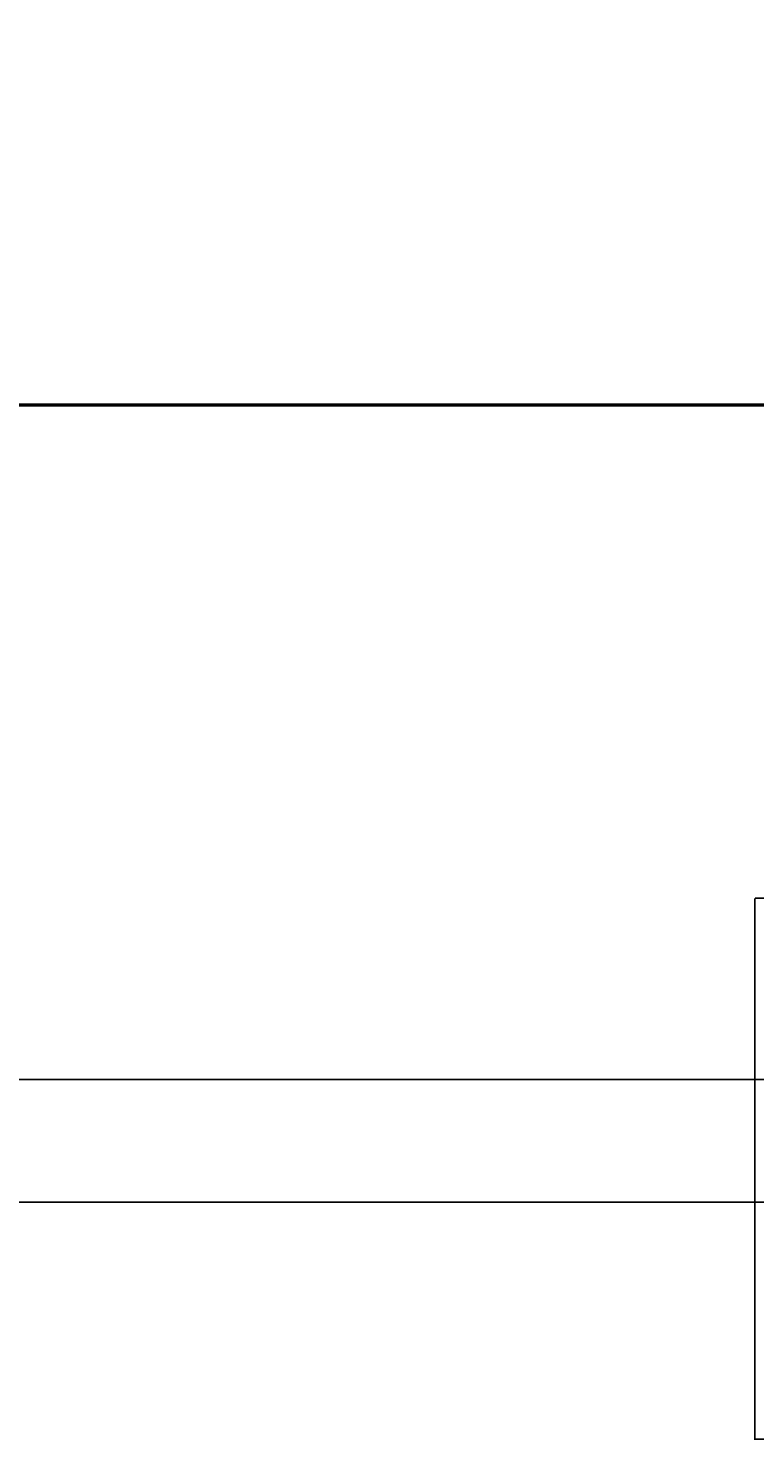
# Model space of a CAD drawing. Units: inches. Extents: x 1693 to 2974, y 2201 to 2965.
# Tile 11 of 24: x 2299 to 2479, y 2201 to 2550. Entities that reach past the tile are written whole.
import ezdxf

# ---------------------------------------------------------------- set-up
doc = ezdxf.new("R2010")
doc.units = ezdxf.units.IN
doc.header["$LTSCALE"] = 2
doc.header["$MEASUREMENT"] = 0
doc.layers.add('A-ANNO-DIMS', color=2, linetype='Continuous', lineweight=18)
doc.styles.get("Standard").update_dxf_attribs({"font": 'arial.ttf'})
doc.dimstyles.get("Standard").update_dxf_attribs({"dimtxt": 0.18, "dimasz": 0.18, "dimexe": 0.18, "dimexo": 0.0625, "dimgap": 0.09, "dimtad": 0, "dimtih": 1, "dimtoh": 1, "dimdec": 1, "dimzin": 0, "dimdsep": 46, "dimlunit": 3, "dimtxsty": 'Standard', "dimcen": 0.09, "dimadec": 0, "dimazin": 0, "dimtfac": 1, "dimtdec": 1, "dimtofl": 0, "dimtmove": 0, "dimatfit": 3, "dimfxl": 1, "dimtolj": 1, "dimtzin": 0, "dimarcsym": 0})

# ---------------------------------------------------------------- blocks, each defined once
blk = doc.blocks.new('*D82')
at = {"layer": 'A-ANNO-DIMS', "color": 0, "lineweight": -2, "ltscale": 2, "transparency": 16777216}
for p, q in [((2615.67, 2906.08), (1693.46, 2906.08)), ((1693.64, 2905.9), (1693.64, 2582.94)), ((1693.64, 2259.62), (1693.64, 2582.58)), ((2096.17, 2259.44), (1693.46, 2259.44))]:
    blk.add_line(p, q, dxfattribs=at)
at = {"layer": 'A-ANNO-DIMS', "color": 0, "ltscale": 2, "transparency": 16777216}
for points in [[(1693.61, 2905.9), (1693.67, 2905.9), (1693.64, 2906.08)], [(1693.61, 2259.62), (1693.67, 2259.62), (1693.64, 2259.44)]]:
    blk.add_solid(points, dxfattribs=at)
at = {"layer": 'Defpoints', "color": 0, "ltscale": 2, "transparency": 16777216}
for p in [(1693.64, 2906.08), (2615.74, 2906.08), (2096.24, 2259.44)]:
    blk.add_point(p, dxfattribs=at)
at = {"layer": 'A-ANNO-DIMS', "color": 0, "ltscale": 2, "transparency": 16777216, "insert": (1693.64, 2582.76), "char_height": 0.18, "attachment_point": 5}
blk.add_mtext('\\A1;646.6', dxfattribs=at)
blk = doc.blocks.new('*D85')
at = {"layer": 'A-ANNO-DIMS', "color": 0, "lineweight": -2, "ltscale": 2, "transparency": 16777216}
for p, q in [((2479.24, 2334.69), (2479.24, 2200.56)), ((2902.24, 2334.69), (2902.24, 2200.56)), ((2479.42, 2200.74), (2690.44, 2200.74)), ((2902.06, 2200.74), (2691.03, 2200.74))]:
    blk.add_line(p, q, dxfattribs=at)
at = {"layer": 'A-ANNO-DIMS', "color": 0, "ltscale": 2, "transparency": 16777216}
for points in [[(2479.42, 2200.77), (2479.42, 2200.71), (2479.24, 2200.74)], [(2902.06, 2200.77), (2902.06, 2200.71), (2902.24, 2200.74)]]:
    blk.add_solid(points, dxfattribs=at)
at = {"layer": 'Defpoints', "color": 0, "ltscale": 2, "transparency": 16777216}
for p in [(2479.24, 2334.75), (2902.24, 2334.75), (2902.24, 2200.74)]:
    blk.add_point(p, dxfattribs=at)
at = {"layer": 'A-ANNO-DIMS', "color": 0, "ltscale": 2, "transparency": 16777216, "insert": (2690.74, 2200.74), "char_height": 0.18, "attachment_point": 5}
blk.add_mtext('\\A1;423', dxfattribs=at)
blk = doc.blocks.new('*D89')
at = {"layer": 'A-ANNO-DIMS', "color": 0, "lineweight": -2, "ltscale": 2, "transparency": 16777216}
for p, q in [((2479.3, 2334.75), (2973.12, 2334.75)), ((2972.94, 2334.57), (2972.94, 2312.48)), ((2972.94, 2290.02), (2972.94, 2312.12)), ((2294.3, 2289.84), (2973.12, 2289.84))]:
    blk.add_line(p, q, dxfattribs=at)
at = {"layer": 'A-ANNO-DIMS', "color": 0, "ltscale": 2, "transparency": 16777216}
for points in [[(2972.91, 2334.57), (2972.97, 2334.57), (2972.94, 2334.75)], [(2972.91, 2290.02), (2972.97, 2290.02), (2972.94, 2289.84)]]:
    blk.add_solid(points, dxfattribs=at)
at = {"layer": 'Defpoints', "color": 0, "ltscale": 2, "transparency": 16777216}
for p in [(2479.24, 2334.75), (2972.94, 2334.75), (2294.24, 2289.84)]:
    blk.add_point(p, dxfattribs=at)
at = {"layer": 'A-ANNO-DIMS', "color": 0, "ltscale": 2, "transparency": 16777216, "insert": (2972.94, 2312.3), "char_height": 0.18, "attachment_point": 5}
blk.add_mtext('\\A1;44.91', dxfattribs=at)
blk = doc.blocks.new('*D95')
at = {"layer": 'A-ANNO-DIMS', "color": 0, "lineweight": -2, "ltscale": 2, "transparency": 16777216}
for p, q in [((2189.3, 2289.84), (2973.12, 2289.84)), ((2972.94, 2289.66), (2972.94, 2274.83)), ((2972.94, 2259.62), (2972.94, 2274.46)), ((2189.3, 2259.44), (2973.12, 2259.44))]:
    blk.add_line(p, q, dxfattribs=at)
at = {"layer": 'A-ANNO-DIMS', "color": 0, "ltscale": 2, "transparency": 16777216}
for points in [[(2972.91, 2289.66), (2972.97, 2289.66), (2972.94, 2289.84)], [(2972.91, 2259.62), (2972.97, 2259.62), (2972.94, 2259.44)]]:
    blk.add_solid(points, dxfattribs=at)
at = {"layer": 'Defpoints', "color": 0, "ltscale": 2, "transparency": 16777216}
for p in [(2189.24, 2289.84), (2972.94, 2289.84), (2189.24, 2259.44)]:
    blk.add_point(p, dxfattribs=at)
at = {"layer": 'A-ANNO-DIMS', "color": 0, "ltscale": 2, "transparency": 16777216, "insert": (2972.94, 2274.64), "char_height": 0.18, "attachment_point": 5}
blk.add_mtext('\\A1;30.4', dxfattribs=at)
blk = doc.blocks.new('*D108')
at = {"layer": 'A-ANNO-DIMS', "color": 0, "lineweight": -2, "ltscale": 2, "transparency": 16777216}
for p, q in [((1752.74, 2457.09), (2973.12, 2457.09)), ((1752.74, 2456.73), (2973.12, 2456.73)), ((2972.94, 2457.27), (2972.94, 2457.45)), ((2972.94, 2457.45), (2973.12, 2457.45)), ((2972.94, 2456.55), (2972.94, 2456.37))]:
    blk.add_line(p, q, dxfattribs=at)
at = {"layer": 'A-ANNO-DIMS', "color": 0, "ltscale": 2, "transparency": 16777216}
for points in [[(2972.91, 2457.27), (2972.97, 2457.27), (2972.94, 2457.09)], [(2972.91, 2456.55), (2972.97, 2456.55), (2972.94, 2456.73)]]:
    blk.add_solid(points, dxfattribs=at)
at = {"layer": 'Defpoints', "color": 0, "ltscale": 2, "transparency": 16777216}
for p in [(1752.68, 2457.09), (1752.68, 2456.73), (2972.94, 2457.09)]:
    blk.add_point(p, dxfattribs=at)
at = {"layer": 'A-ANNO-DIMS', "color": 0, "ltscale": 2, "transparency": 16777216, "insert": (2973.44, 2457.45), "char_height": 0.18, "attachment_point": 5}
blk.add_mtext('\\A1;0.36', dxfattribs=at)

msp = doc.modelspace()

# ---------------------------------------------------------------- dimensions: what is measured, and where the dimension line sits
at = {"layer": 'A-ANNO-DIMS', "ltscale": 2}
for base, p1, p2, override, picture, middle in [((1693.6363, 2906.0761), (2096.2363, 2259.4449), (2615.7363, 2906.0761), {"dimdec": 1, "dimlfac": 1, "dimrnd": 0, "dimzin": 0, "dimdsep": 46, "dimlunit": 2}, '*D82', (1693.6363, 2582.7605)), ((2972.9363, 2457.0877), (1752.6754, 2456.7302), (1752.6754, 2457.0877), {"dimdec": 2, "dimlfac": 1, "dimrnd": 0, "dimzin": 0, "dimdsep": 46, "dimlunit": 2}, '*D108', (2973.44, 2457.4477)), ((2972.9363, 2334.7547), (2294.2363, 2289.8449), (2479.2363, 2334.7547), {"dimdec": 2, "dimlfac": 1, "dimrnd": 0, "dimzin": 0, "dimdsep": 46, "dimlunit": 2}, '*D89', (2972.9363, 2312.2998)), ((2972.9363, 2289.8449), (2189.2363, 2259.4449), (2189.2363, 2289.8449), {"dimdec": 1, "dimlfac": 1, "dimrnd": 0, "dimzin": 0, "dimdsep": 46, "dimlunit": 2}, '*D95', (2972.9363, 2274.6449))]:
    dim = msp.add_linear_dim(base=base, p1=p1, p2=p2, angle=90, dimstyle='Standard', override=override, dxfattribs=at)
    dim.commit()
    dim.dimension.update_dxf_attribs({"geometry": picture, "text_midpoint": middle})
dim = msp.add_linear_dim(base=(2902.2363, 2200.7449), p1=(2479.2363, 2334.7547), p2=(2902.2363, 2334.7547), dimstyle='Standard', override={"dimdec": 0, "dimlfac": 1, "dimrnd": 0, "dimzin": 0, "dimdsep": 46, "dimlunit": 2}, dxfattribs=at)
dim.commit()
dim.dimension.update_dxf_attribs({"geometry": '*D85', "text_midpoint": (2690.7363, 2200.7449)})

doc.saveas('drawing.dxf')
